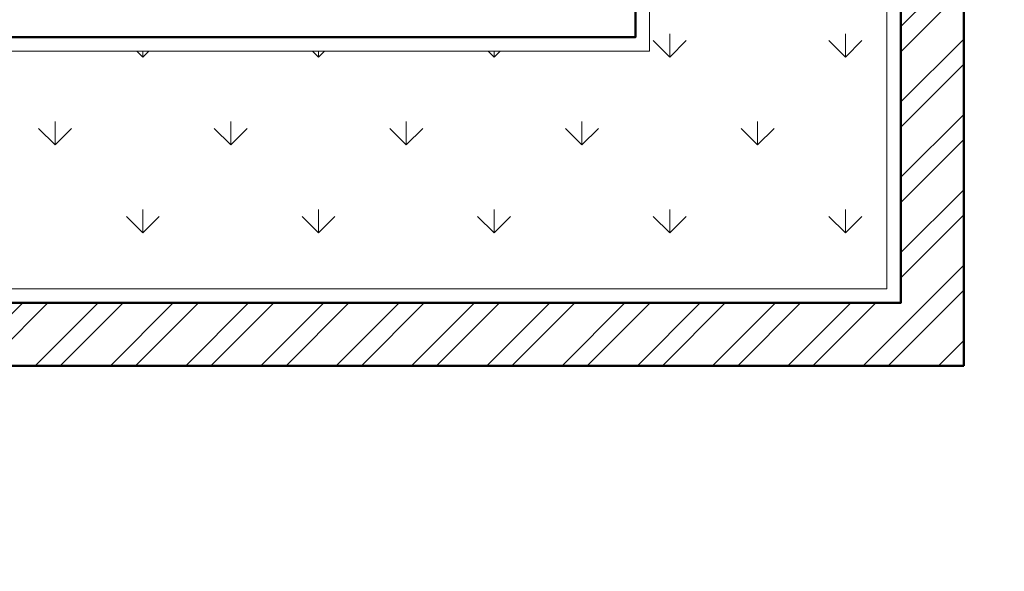
# Model space of a CAD drawing. Units: inches. Extents: x 261 to 2725, y 291 to 1454.
# Tile 30 of 35: x 2359 to 2500, y 467 to 546. Entities that reach past the tile are written whole.
import ezdxf

# ---------------------------------------------------------------- set-up
doc = ezdxf.new("R2010")
doc.units = ezdxf.units.IN
for name, color, linetype, lineweight in [('A-ANNO-DIMS', 136, 'Continuous', 18), ('A-PLNT', 3, 'Continuous', 18), ('A-PLNT-PATT', 3, 'Continuous', 13), ('A-WALL', 222, 'Continuous', 50), ('A-WALL-PATT', 243, 'Continuous', 13)]:
    doc.layers.add(name, color=color, linetype=linetype, lineweight=lineweight)
doc.styles.get("Standard").update_dxf_attribs({"font": 'arial.ttf'})
doc.dimstyles.new('ISO-25', dxfattribs={"dimtxt": 12, "dimasz": 6, "dimexe": 1.25, "dimexo": 0.625, "dimtad": 1, "dimdec": 0, "dimlunit": 3, "dimtxsty": 'Standard', "dimblk": 'ARCHTICK', "dimcen": 2.5, "dimadec": 0, "dimazin": 0, "dimtfac": 1, "dimtdec": 0, "dimtmove": 0, "dimatfit": 3, "dimfxl": 1, "dimfxlon": 1, "dimarcsym": 0})

# ---------------------------------------------------------------- blocks, each defined once
blk = doc.blocks.new('_ArchTick')
at = {"color": 0, "linetype": 'ByBlock', "const_width": 0.15}
blk.add_lwpolyline([(-0.5, -0.5), (0.5, 0.5)], dxfattribs=at)
blk = doc.blocks.new('*D82')
at = {"layer": 'A-ANNO-DIMS', "color": 0, "lineweight": -2, "ltscale": 0.07, "transparency": 16777216}
for p, q in [((2600.96, 679.47), (2603.21, 679.47)), ((2601.96, 517.47), (2601.96, 679.47)), ((2600.96, 517.47), (2603.21, 517.47))]:
    blk.add_line(p, q, dxfattribs=at)
at = {"layer": 'Defpoints', "color": 0, "ltscale": 0.07, "transparency": 16777216}
for p in [(946.45, 679.47), (2601.96, 679.47), (946.45, 517.47)]:
    blk.add_point(p, dxfattribs=at)
at = {"layer": 'A-ANNO-DIMS', "color": 0, "lineweight": -2, "ltscale": 0.07, "transparency": 16777216, "xscale": 6, "yscale": 6, "zscale": 6}
for p, rotation in [((2601.96, 679.47), 90), ((2601.96, 517.47), 270)]:
    blk.add_blockref('_ArchTick', p, dxfattribs=dict(at, rotation=rotation))
at = {"layer": 'A-ANNO-DIMS', "color": 0, "ltscale": 0.07, "transparency": 16777216, "insert": (2595.2, 598.47), "char_height": 12, "attachment_point": 5, "rotation": 90}
blk.add_mtext('13\'-6"', dxfattribs=at)
blk = doc.blocks.new('*D89')
at = {"layer": 'A-ANNO-DIMS', "color": 0, "lineweight": -2, "ltscale": 0.07, "transparency": 16777216}
for p, q in [((2600.96, 508.47), (2603.21, 508.47)), ((2601.96, 412.47), (2601.96, 508.47)), ((2600.96, 412.47), (2603.21, 412.47))]:
    blk.add_line(p, q, dxfattribs=at)
at = {"layer": 'Defpoints', "color": 0, "ltscale": 0.07, "transparency": 16777216}
for p in [(955.45, 508.47), (2601.96, 508.47), (994.45, 412.47)]:
    blk.add_point(p, dxfattribs=at)
at = {"layer": 'A-ANNO-DIMS', "color": 0, "lineweight": -2, "ltscale": 0.07, "transparency": 16777216, "xscale": 6, "yscale": 6, "zscale": 6}
for p, rotation in [((2601.96, 508.47), 90), ((2601.96, 412.47), 270)]:
    blk.add_blockref('_ArchTick', p, dxfattribs=dict(at, rotation=rotation))
at = {"layer": 'A-ANNO-DIMS', "color": 0, "ltscale": 0.07, "transparency": 16777216, "insert": (2595.21, 460.47), "char_height": 12, "attachment_point": 5, "rotation": 90}
blk.add_mtext('8\'-0"', dxfattribs=at)
blk = doc.blocks.new('*D111')
at = {"layer": 'A-ANNO-DIMS', "color": 0, "lineweight": -2, "ltscale": 0.07, "transparency": 16777216}
for p, q in [((2600.96, 550.47), (2603.21, 550.47)), ((2601.96, 448.47), (2601.96, 550.47)), ((2600.96, 448.47), (2603.21, 448.47))]:
    blk.add_line(p, q, dxfattribs=at)
at = {"layer": 'Defpoints', "color": 0, "ltscale": 0.07, "transparency": 16777216}
for p in [(1720.08, 550.47), (2601.96, 550.47), (1720.08, 448.47)]:
    blk.add_point(p, dxfattribs=at)
at = {"layer": 'A-ANNO-DIMS', "color": 0, "lineweight": -2, "ltscale": 0.07, "transparency": 16777216, "xscale": 6, "yscale": 6, "zscale": 6}
for p, rotation in [((2601.96, 550.47), 90), ((2601.96, 448.47), 270)]:
    blk.add_blockref('_ArchTick', p, dxfattribs=dict(at, rotation=rotation))
at = {"layer": 'A-ANNO-DIMS', "color": 0, "ltscale": 0.07, "transparency": 16777216, "insert": (2595.21, 499.47), "char_height": 12, "attachment_point": 5, "rotation": 90}
blk.add_mtext('8\'-6"', dxfattribs=at)
blk = doc.blocks.new('*D125')
at = {"layer": 'A-ANNO-DIMS', "color": 0, "lineweight": -2, "ltscale": 0.07, "transparency": 16777216}
for p, q in [((2600.96, 496.47), (2603.21, 496.47)), ((2601.96, 439.47), (2601.96, 496.47)), ((2600.96, 439.47), (2603.21, 439.47))]:
    blk.add_line(p, q, dxfattribs=at)
at = {"layer": 'Defpoints', "color": 0, "ltscale": 0.07, "transparency": 16777216}
for p in [(2214.67, 496.47), (2601.96, 496.47), (2214.67, 439.47)]:
    blk.add_point(p, dxfattribs=at)
at = {"layer": 'A-ANNO-DIMS', "color": 0, "lineweight": -2, "ltscale": 0.07, "transparency": 16777216, "xscale": 6, "yscale": 6, "zscale": 6}
for p, rotation in [((2601.96, 496.47), 90), ((2601.96, 439.47), 270)]:
    blk.add_blockref('_ArchTick', p, dxfattribs=dict(at, rotation=rotation))
at = {"layer": 'A-ANNO-DIMS', "color": 0, "ltscale": 0.07, "transparency": 16777216, "insert": (2595.21, 467.97), "char_height": 12, "attachment_point": 5, "rotation": 90}
blk.add_mtext('4\'-9"', dxfattribs=at)
blk = doc.blocks.new('*D126')
at = {"layer": 'A-ANNO-DIMS', "color": 0, "lineweight": -2, "ltscale": 0.07, "transparency": 16777216}
for p, q in [((2600.96, 673.47), (2603.21, 673.47)), ((2601.96, 496.47), (2601.96, 673.47)), ((2600.96, 496.47), (2603.21, 496.47))]:
    blk.add_line(p, q, dxfattribs=at)
at = {"layer": 'Defpoints', "color": 0, "ltscale": 0.07, "transparency": 16777216}
for p in [(2484.71, 673.47), (2601.96, 673.47), (2493.71, 496.47)]:
    blk.add_point(p, dxfattribs=at)
at = {"layer": 'A-ANNO-DIMS', "color": 0, "lineweight": -2, "ltscale": 0.07, "transparency": 16777216, "xscale": 6, "yscale": 6, "zscale": 6}
for p, rotation in [((2601.96, 673.47), 90), ((2601.96, 496.47), 270)]:
    blk.add_blockref('_ArchTick', p, dxfattribs=dict(at, rotation=rotation))
at = {"layer": 'A-ANNO-DIMS', "color": 0, "ltscale": 0.07, "transparency": 16777216, "insert": (2595.21, 584.97), "char_height": 12, "attachment_point": 5, "rotation": 90}
blk.add_mtext('14\'-9"', dxfattribs=at)
blk = doc.blocks.new('*D130')
at = {"layer": 'A-ANNO-DIMS', "color": 0, "lineweight": -2, "ltscale": 0.07, "transparency": 16777216}
for p, q in [((2600.96, 541.47), (2603.21, 541.47)), ((2601.96, 505.47), (2601.96, 541.47)), ((2600.96, 505.47), (2603.21, 505.47))]:
    blk.add_line(p, q, dxfattribs=at)
at = {"layer": 'Defpoints', "color": 0, "ltscale": 0.07, "transparency": 16777216}
for p in [(2448.71, 541.47), (2601.96, 541.47), (2484.71, 505.47)]:
    blk.add_point(p, dxfattribs=at)
at = {"layer": 'A-ANNO-DIMS', "color": 0, "lineweight": -2, "ltscale": 0.07, "transparency": 16777216, "xscale": 6, "yscale": 6, "zscale": 6}
for p, rotation in [((2601.96, 541.47), 90), ((2601.96, 505.47), 270)]:
    blk.add_blockref('_ArchTick', p, dxfattribs=dict(at, rotation=rotation))
at = {"layer": 'A-ANNO-DIMS', "color": 0, "ltscale": 0.07, "transparency": 16777216, "insert": (2595.2, 523.47), "char_height": 12, "attachment_point": 5, "rotation": 90}
blk.add_mtext('3\'-0"', dxfattribs=at)
blk = doc.blocks.new('*D131')
at = {"layer": 'A-ANNO-DIMS', "color": 0, "lineweight": -2, "ltscale": 0.07, "transparency": 16777216}
for p, q in [((2448.71, 305.22), (2448.71, 302.97)), ((2484.71, 305.22), (2484.71, 302.97)), ((2448.71, 304.22), (2484.71, 304.22))]:
    blk.add_line(p, q, dxfattribs=at)
at = {"layer": 'Defpoints', "color": 0, "ltscale": 0.07, "transparency": 16777216}
for p in [(2484.71, 673.47), (2448.71, 671.47), (2484.71, 304.22)]:
    blk.add_point(p, dxfattribs=at)
at = {"layer": 'A-ANNO-DIMS', "color": 0, "lineweight": -2, "ltscale": 0.07, "transparency": 16777216, "xscale": 6, "yscale": 6, "zscale": 6, "rotation": 180}
blk.add_blockref('_ArchTick', (2448.71, 304.22), dxfattribs=at)
at = {"layer": 'A-ANNO-DIMS', "color": 0, "lineweight": -2, "ltscale": 0.07, "transparency": 16777216, "xscale": 6, "yscale": 6, "zscale": 6}
blk.add_blockref('_ArchTick', (2484.71, 304.22), dxfattribs=at)
at = {"layer": 'A-ANNO-DIMS', "color": 0, "ltscale": 0.07, "transparency": 16777216, "insert": (2466.71, 310.97), "char_height": 12, "attachment_point": 5}
blk.add_mtext('3\'-0"', dxfattribs=at)
blk = doc.blocks.new('*D132')
at = {"layer": 'A-ANNO-DIMS', "color": 0, "lineweight": -2, "ltscale": 0.07, "transparency": 16777216}
for p, q in [((2364.21, 305.22), (2364.21, 302.97)), ((2484.71, 305.22), (2484.71, 302.97)), ((2364.21, 304.22), (2484.71, 304.22))]:
    blk.add_line(p, q, dxfattribs=at)
at = {"layer": 'Defpoints', "color": 0, "ltscale": 0.07, "transparency": 16777216}
for p in [(2364.21, 799.47), (2484.71, 799.47), (2484.71, 304.22)]:
    blk.add_point(p, dxfattribs=at)
at = {"layer": 'A-ANNO-DIMS', "color": 0, "lineweight": -2, "ltscale": 0.07, "transparency": 16777216, "xscale": 6, "yscale": 6, "zscale": 6, "rotation": 180}
blk.add_blockref('_ArchTick', (2364.21, 304.22), dxfattribs=at)
at = {"layer": 'A-ANNO-DIMS', "color": 0, "lineweight": -2, "ltscale": 0.07, "transparency": 16777216, "xscale": 6, "yscale": 6, "zscale": 6}
blk.add_blockref('_ArchTick', (2484.71, 304.22), dxfattribs=at)
at = {"layer": 'A-ANNO-DIMS', "color": 0, "ltscale": 0.07, "transparency": 16777216, "insert": (2424.46, 311.05), "char_height": 12, "attachment_point": 5}
blk.add_mtext('10\'-0 1/2"', dxfattribs=at)
blk = doc.blocks.new('*D136')
at = {"layer": 'A-ANNO-DIMS', "color": 0, "lineweight": -2, "ltscale": 0.07, "transparency": 16777216}
for p, q in [((2600.96, 675.78), (2603.21, 675.78)), ((2601.96, 675.78), (2601.96, 475.47)), ((2600.96, 475.47), (2603.21, 475.47))]:
    blk.add_line(p, q, dxfattribs=at)
at = {"layer": 'Defpoints', "color": 0, "ltscale": 0.07, "transparency": 16777216}
for p in [(2208.67, 675.78), (2208.67, 475.47), (2601.96, 475.47)]:
    blk.add_point(p, dxfattribs=at)
at = {"layer": 'A-ANNO-DIMS', "color": 0, "lineweight": -2, "ltscale": 0.07, "transparency": 16777216, "xscale": 6, "yscale": 6, "zscale": 6}
for p, rotation in [((2601.96, 675.78), 90), ((2601.96, 475.47), 270)]:
    blk.add_blockref('_ArchTick', p, dxfattribs=dict(at, rotation=rotation))
at = {"layer": 'A-ANNO-DIMS', "color": 0, "ltscale": 0.07, "transparency": 16777216, "insert": (2595.13, 575.62), "char_height": 12, "attachment_point": 5, "rotation": 90}
blk.add_mtext('16\'-8 1/2"', dxfattribs=at)
blk = doc.blocks.new('*D138')
at = {"layer": 'A-ANNO-DIMS', "color": 0, "lineweight": -2, "ltscale": 0.07, "transparency": 16777216}
for p, q in [((2600.96, 634.05), (2603.21, 634.05)), ((2601.96, 634.05), (2601.96, 517.2)), ((2600.96, 517.2), (2603.21, 517.2))]:
    blk.add_line(p, q, dxfattribs=at)
at = {"layer": 'Defpoints', "color": 0, "ltscale": 0.07, "transparency": 16777216}
for p in [(2221.19, 634.05), (2221.19, 517.2), (2601.96, 517.2)]:
    blk.add_point(p, dxfattribs=at)
at = {"layer": 'A-ANNO-DIMS', "color": 0, "lineweight": -2, "ltscale": 0.07, "transparency": 16777216, "xscale": 6, "yscale": 6, "zscale": 6}
for p, rotation in [((2601.96, 634.05), 90), ((2601.96, 517.2), 270)]:
    blk.add_blockref('_ArchTick', p, dxfattribs=dict(at, rotation=rotation))
at = {"layer": 'A-ANNO-DIMS', "color": 0, "ltscale": 0.07, "transparency": 16777216, "insert": (2595.21, 575.62), "char_height": 12, "attachment_point": 5, "rotation": 90}
blk.add_mtext('9\'-9"', dxfattribs=at)

msp = doc.modelspace()

# ---------------------------------------------------------------- hatches: boundary and pattern name
at = {"layer": 'A-PLNT-PATT'}
h = msp.add_hatch(dxfattribs=at)
h.set_pattern_fill('GRASS', color=256, scale=0.7)
h.paths.add_polyline_path([(2052.71, 797.47), (2018.71, 797.47), (2018.71, 450.47), (2206.67, 450.47), (2206.67, 507.47), (2482.71, 507.47), (2482.71, 671.47), (2448.71, 671.47), (2448.71, 541.47), (2172.67, 541.47), (2172.67, 484.47), (2052.71, 484.47)])
at = {"layer": 'A-WALL-PATT'}
h = msp.add_hatch(dxfattribs=at)
h.set_pattern_fill('ANSI32', color=256, scale=0.8)
h.paths.add_polyline_path([(478.45, 685.47), (580.45, 685.47), (580.45, 691.47), (577.45, 691.47), (577.45, 694.47), (571.45, 694.47), (571.45, 691.47), (478.45, 691.47), (478.45, 721.47), (469.45, 721.47), (469.45, 508.47), (538.45, 508.47), (538.45, 517.47), (478.45, 517.47)])
h.paths.add_polyline_path([(694.45, 517.47), (676.45, 517.47), (676.45, 646.47), (670.45, 646.47), (670.45, 517.47), (610.45, 517.47), (610.45, 508.47), (694.45, 508.47)])
h.paths.add_polyline_path([(676.45, 784.47), (478.45, 784.47), (478.45, 844.47), (469.45, 844.47), (469.45, 745.47), (478.45, 745.47), (478.45, 775.47), (571.45, 775.47), (571.45, 724.47), (577.45, 724.47), (577.45, 775.47), (670.45, 775.47), (670.45, 691.47), (610.45, 691.47), (610.45, 685.47), (670.45, 685.47), (670.45, 682.47), (676.45, 682.47)])
h.paths.add_polyline_path([(955.45, 880.47), (946.45, 880.47), (946.45, 808.47), (778.45, 808.47), (778.45, 799.47), (946.45, 799.47), (946.45, 517.47), (898.45, 517.47), (898.45, 508.47), (955.45, 508.47)])
h.paths.add_polyline_path([(778.45, 598.47), (772.45, 598.47), (772.45, 517.47), (754.45, 517.47), (754.45, 508.47), (826.45, 508.47), (826.45, 517.47), (778.45, 517.47)])
h.paths.add_polyline_path([(955.45, 1090.47), (946.45, 1090.47), (946.45, 1030.47), (817.45, 1030.47), (817.45, 1024.47), (946.45, 1024.47), (946.45, 952.47), (955.45, 952.47)])
h.paths.add_polyline_path([(955.45, 1231.47), (730.45, 1231.47), (730.45, 1222.47), (772.45, 1222.47), (772.45, 1096.47), (766.45, 1096.47), (766.45, 1090.47), (772.45, 1090.47), (772.45, 1006.47), (712.45, 1006.47), (712.45, 1000.47), (778.45, 1000.47), (778.45, 1024.47), (781.45, 1024.47), (781.45, 1030.47), (778.45, 1030.47), (778.45, 1222.47), (946.45, 1222.47), (946.45, 1162.47), (955.45, 1162.47)])
h.paths.add_polyline_path([(694.45, 1231.47), (619.45, 1231.47), (619.45, 1222.47), (646.45, 1222.47), (646.45, 1039.47), (652.45, 1039.47), (652.45, 1090.47), (736.45, 1090.47), (736.45, 1096.47), (652.45, 1096.47), (652.45, 1222.47), (694.45, 1222.47)])
h.paths.add_polyline_path([(571.45, 1231.47), (469.45, 1231.47), (469.45, 1099.47), (478.45, 1099.47), (478.45, 1144.47), (544.45, 1144.47), (544.45, 1153.47), (538.45, 1153.47), (538.45, 1150.47), (478.45, 1150.47), (478.45, 1222.47), (538.45, 1222.47), (538.45, 1183.47), (544.45, 1183.47), (544.45, 1222.47), (571.45, 1222.47)])
h.paths.add_polyline_path([(538.45, 1006.47), (478.45, 1006.47), (478.45, 1051.47), (469.45, 1051.47), (469.45, 940.47), (478.45, 940.47), (478.45, 1000.47), (538.45, 1000.47)])
h.paths.add_polyline_path([(652.45, 1006.47), (652.45, 1009.47), (646.45, 1009.47), (646.45, 1006.47), (586.45, 1006.47), (586.45, 1000.47), (652.45, 1000.47)])
h.paths.add_polyline_path([(1288.08, 973.47), (1243.08, 973.47), (1243.08, 920.97), (1252.08, 920.97), (1252.08, 964.47), (1288.08, 964.47)], flags=17)
h.paths.add_polyline_path([(1402.08, 805.47), (1252.08, 805.47), (1252.08, 848.97), (1243.08, 848.97), (1243.08, 757.47), (1252.08, 757.47), (1252.08, 799.47), (1294.08, 799.47), (1372.08, 799.47), (1372.08, 779.47), (1372.08, 715.47), (1378.08, 715.47), (1378.08, 799.47), (1402.08, 799.47)])
h.paths.add_polyline_path([(1252.08, 721.47), (1243.08, 721.47), (1243.08, 439.47), (1729.08, 439.47), (1729.08, 709.47), (1720.08, 709.47), (1720.08, 679.47), (1582.08, 679.47), (1582.08, 670.47), (1588.08, 670.47), (1588.08, 673.47), (1720.08, 673.47), (1720.08, 559.47), (1690.08, 559.47), (1690.08, 550.47), (1720.08, 550.47), (1720.08, 448.47), (1252.08, 448.47), (1252.08, 496.47), (1312.08, 496.47), (1312.08, 505.47), (1252.08, 505.47), (1252.08, 673.47), (1405.08, 673.47), (1405.08, 679.47), (1378.08, 679.47), (1378.08, 685.47), (1372.08, 685.47), (1372.08, 679.47), (1252.08, 679.47)])
h.paths.add_polyline_path([(1450.08, 550.47), (1480.08, 550.47), (1480.08, 559.47), (1450.08, 559.47), (1450.08, 679.47), (1441.08, 679.47), (1441.08, 673.47), (1444.08, 673.47), (1444.08, 505.47), (1384.08, 505.47), (1384.08, 496.47), (1450.08, 496.47)], flags=17)
h.paths.add_polyline_path([(1618.08, 559.47), (1588.08, 559.47), (1588.08, 634.47), (1582.08, 634.47), (1582.08, 559.47), (1552.08, 559.47), (1552.08, 550.47), (1618.08, 550.47)], flags=17)
h.paths.add_polyline_path([(1564.08, 964.47), (1630.08, 964.47), (1630.08, 973.47), (1477.08, 973.47), (1477.08, 964.47), (1558.08, 964.47), (1558.08, 926.22), (1558.08, 887.97), (1486.08, 887.97), (1486.08, 881.97), (1558.08, 881.97), (1558.08, 805.47), (1450.08, 805.47), (1450.08, 845.97), (1444.08, 845.97), (1444.08, 805.47), (1438.08, 805.47), (1438.08, 799.47), (1564.08, 799.47)], flags=17)
h.paths.add_polyline_path([(1453.08, 973.47), (1408.08, 973.47), (1408.08, 964.47), (1444.08, 964.47), (1444.08, 881.97), (1450.08, 881.97), (1456.08, 881.97), (1456.08, 887.97), (1450.08, 887.97), (1450.08, 964.47), (1453.08, 964.47)], flags=17)
h.paths.add_polyline_path([(1729.08, 1231.47), (1243.08, 1231.47), (1243.08, 1167.47), (1252.08, 1167.47), (1252.08, 1222.47), (1441.08, 1222.47), (1441.08, 1045.47), (1648.08, 1045.47), (1648.08, 1051.47), (1450.08, 1051.47), (1450.08, 1074.47), (1450.08, 1222.47), (1472.08, 1222.47), (1720.08, 1222.47), (1720.08, 1051.47), (1708.08, 1051.47), (1708.08, 1045.47), (1720.08, 1045.47), (1720.08, 973.47), (1702.08, 973.47), (1702.08, 964.47), (1720.08, 964.47), (1720.08, 769.47), (1729.08, 769.47)])
h.paths.add_polyline_path([(2493.71, 1054.85), (2007.71, 1054.85), (2007.71, 439.47), (2214.67, 439.47), (2214.67, 496.47), (2493.71, 496.47)])
h.paths.add_polyline_path([(2016.71, 1045.85), (2304.71, 1045.85), (2304.71, 841.47), (2310.71, 841.47), (2310.71, 1045.85), (2484.71, 1045.85), (2484.71, 805.47), (2310.71, 805.47), (2310.71, 811.47), (2304.71, 811.47), (2304.71, 799.47), (2484.71, 799.47), (2484.71, 679.47), (2304.71, 679.47), (2304.71, 673.47), (2484.71, 673.47), (2484.71, 505.47), (2208.67, 505.47), (2208.67, 448.47), (2016.71, 448.47), (2016.71, 799.47), (2304.71, 799.47), (2304.71, 805.47), (2016.71, 805.47)], flags=16)

# ---------------------------------------------------------------- linework, layer by layer
at = {"layer": 'A-PLNT'}
for points in [[(2018.71, 797.47), (2018.71, 450.47), (2206.67, 450.47), (2206.67, 507.47), (2482.71, 507.47), (2482.71, 671.47)], [(2052.71, 797.47), (2052.71, 484.47), (2172.67, 484.47), (2172.67, 541.47), (2448.71, 541.47), (2448.71, 671.47)]]:
    msp.add_lwpolyline(points, dxfattribs=at)
at = {"layer": 'A-WALL'}
for p in [(2493.71, 1054.85), (2214.67, 496.47)]:
    msp.add_line(p, (2493.71, 496.47), dxfattribs=at)
for points in [[(2016.71, 799.47), (2016.71, 448.47), (2208.67, 448.47), (2208.67, 505.47), (2484.71, 505.47), (2484.71, 673.47)], [(2054.71, 799.47), (2054.71, 486.47), (2170.67, 486.47), (2170.67, 543.47), (2446.71, 543.47), (2446.71, 673.47)]]:
    msp.add_lwpolyline(points, dxfattribs=at)

# ---------------------------------------------------------------- dimensions: what is measured, and where the dimension line sits
at = {"layer": 'A-ANNO-DIMS', "ltscale": 0.07}
for p1, p2, picture, middle in [((2364.21, 799.47), (2484.71, 799.47), '*D132', (2424.46, 311.05)), ((2448.71, 671.47), (2484.71, 673.47), '*D131', (2466.71, 310.97))]:
    dim = msp.add_linear_dim(base=(2484.71, 304.22), p1=p1, p2=p2, dimstyle='ISO-25', override={"dimdec": 1, "dimlfac": 1, "dimrnd": 0, "dimzin": 1, "dimdsep": 46, "dimlunit": 4, "dimfrac": 2}, dxfattribs=at)
    dim.commit()
    dim.dimension.update_dxf_attribs({"geometry": picture, "text_midpoint": middle})
for base, p1, p2, picture, middle in [((2601.96, 679.47), (946.45, 517.47), (946.45, 679.47), '*D82', (2595.2, 598.47)), ((2601.96, 475.47), (2208.67, 675.78), (2208.67, 475.47), '*D136', (2595.13, 575.62)), ((2601.96, 673.47), (2493.71, 496.47), (2484.71, 673.47), '*D126', (2595.21, 584.97)), ((2601.9578, 517.1998), (2221.1928, 634.0483), (2221.1928, 517.1998), '*D138', (2595.2059, 575.6241)), ((2601.96, 550.47), (1720.08, 448.47), (1720.08, 550.47), '*D111', (2595.21, 499.47)), ((2601.96, 541.47), (2484.71, 505.47), (2448.71, 541.47), '*D130', (2595.2, 523.47)), ((2601.96, 508.47), (994.45, 412.47), (955.45, 508.47), '*D89', (2595.21, 460.47)), ((2601.96, 496.47), (2214.67, 439.47), (2214.67, 496.47), '*D125', (2595.21, 467.97))]:
    dim = msp.add_linear_dim(base=base, p1=p1, p2=p2, angle=90, dimstyle='ISO-25', override={"dimdec": 1, "dimlfac": 1, "dimrnd": 0, "dimzin": 1, "dimdsep": 46, "dimlunit": 4, "dimfrac": 2}, dxfattribs=at)
    dim.commit()
    dim.dimension.update_dxf_attribs({"geometry": picture, "text_midpoint": middle})

doc.saveas('drawing.dxf')
